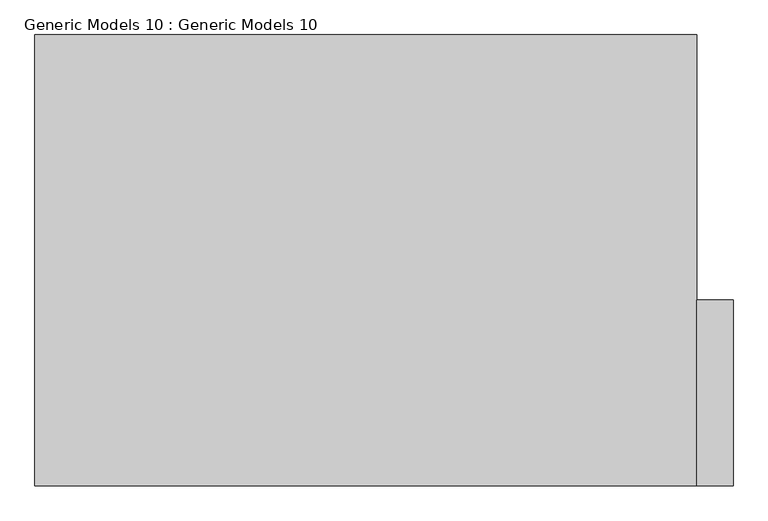
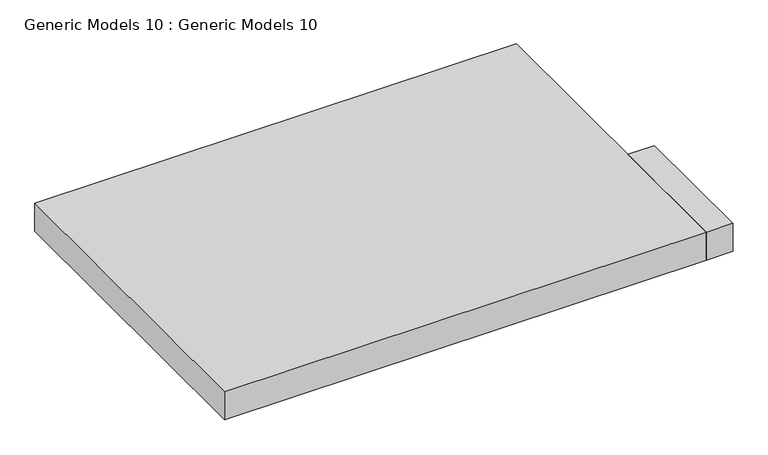
"""IFC4 building model written with IfcOpenShell, lengths in millimetres: proxy geometry, Generic Models 10 : Generic Models 10."""

from ifc_helpers import new_model, si_unit, frame, origin, place, context, project, spatial, polyline, outline, extrude, source, transform, mapped, element, save


def generic_models_10_generic_models_10_b7097970(model_context):
    return source(origin(), model_context, "Body", "SweptSolid", [
        extrude(outline(polyline([(-10521.0371373, -2516.661407), (-10521.0371373, -3685.061407), (-10749.6371373, -3685.061407), (-10749.6371373, -2516.661407), (-10521.0371373, -2516.661407)])), frame((0.0, 0.0, 3098.8), z_axis=(0.0, 0.0, 1.0), x_axis=(1.0, 0.0, 0.0)), (0.0, 0.0, 1.0), 254.0),
        extrude(outline(polyline([(-10749.6371373, -852.961407), (-10749.6371373, -3685.061407), (-14902.5371373, -3685.061407), (-14902.5371373, -852.961407), (-10749.6371373, -852.961407)])), frame((0.0, 0.0, 3098.8), z_axis=(0.0, 0.0, 1.0), x_axis=(1.0, 0.0, 0.0)), (0.0, 0.0, 1.0), 254.0),
    ])


if __name__ == "__main__":
    model = new_model("IFC4")
    model_context = context("Model", 3, world=origin())
    ifc_project = project(units=[si_unit("LENGTHUNIT", "METRE", prefix="MILLI")], contexts=[model_context])
    site = spatial("IfcSite", under=ifc_project)
    building = spatial("IfcBuilding", under=site)
    placement = place(None, origin())
    generic_models_10_generic_models_10_shape = generic_models_10_generic_models_10_b7097970(model_context)
    element("IfcBuildingElementProxy", 1, Name="Generic Models 10 : Generic Models 10", ObjectType="Generic Models 10 : Generic Models 10", at=placement, inside=building, context=model_context, shape_type="MappedRepresentation", body=[
        mapped(generic_models_10_generic_models_10_shape, transform((0.0, 0.0, 0.0), x_axis=(1.0, 0.0, 0.0), y_axis=(0.0, 1.0, 0.0), z_axis=(0.0, 0.0, 1.0))),
    ])
    save(model, "model.ifc")

# Revit data of these elements
# Element 1 (IfcBuildingElementProxy, "Generic Models 10 : Generic Models 10")
#   Materials on its faces: "Gypsum Wall Board"
# Materials
#   "Gypsum Wall Board": class "Generic", colour RGB 127 127 127, transparency 0, Description = "Gypsum Wall Board", Cost = 0
